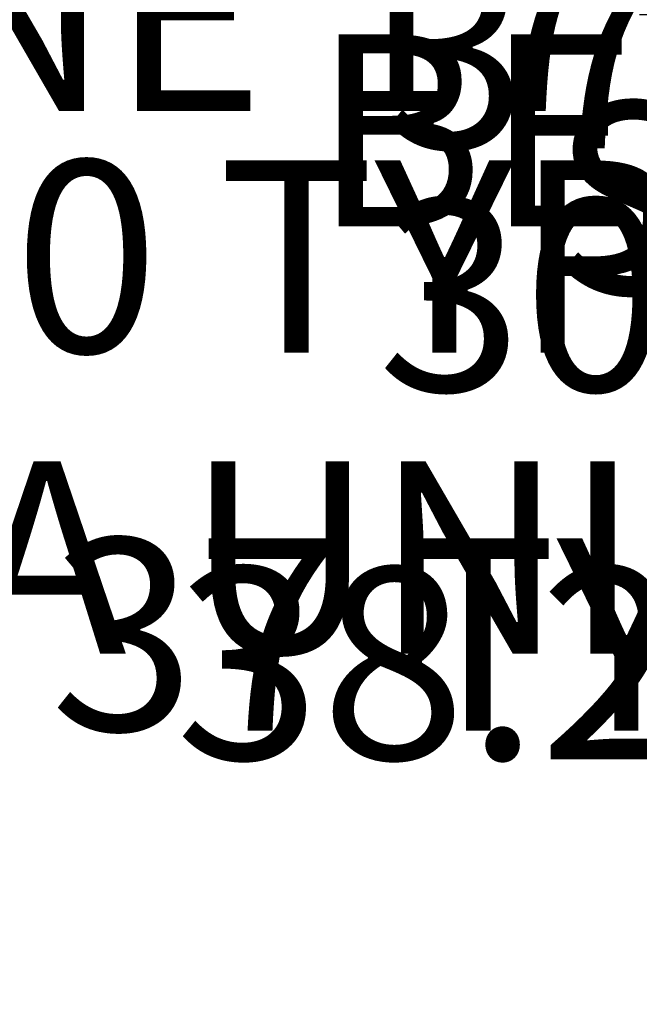
# Model space of a CAD drawing. Units: inches. Extents: x -307 to 2141, y -58 to 895.
# Tile 2 of 28: x 237 to 469, y -58 to 312. Entities that reach past the tile are written whole.
import ezdxf

# ---------------------------------------------------------------- set-up
doc = ezdxf.new("R2010")
doc.units = ezdxf.units.IN
doc.header["$MEASUREMENT"] = 0
doc.layers.add('A-ANNO-DIMS', color=2, linetype='Continuous', lineweight=18)
doc.styles.get("Standard").update_dxf_attribs({"font": 'arial.ttf'})
doc.dimstyles.get("Standard").update_dxf_attribs({"dimtxt": 72, "dimasz": 48, "dimexe": 0.18, "dimexo": 0.0625, "dimgap": 0.09, "dimtad": 0, "dimtih": 1, "dimtoh": 1, "dimdec": 0, "dimrnd": 48, "dimzin": 0, "dimdsep": 46, "dimlunit": 3, "dimtxsty": 'Standard', "dimcen": 0.09, "dimadec": 0, "dimazin": 0, "dimtfac": 1, "dimtdec": 0, "dimtofl": 0, "dimtmove": 0, "dimatfit": 3, "dimfxl": 1, "dimtolj": 1, "dimtzin": 0, "dimarcsym": 0})

# ---------------------------------------------------------------- blocks, each defined once
blk = doc.blocks.new('*D28')
at = {"layer": 'A-ANNO-DIMS', "color": 0, "lineweight": -2, "transparency": 16777216}
for p, q in [((795.36, 433.55), (777.92, 433.55)), ((778.1, 385.55), (778.1, 366.07)), ((795.36, 318.07), (777.92, 318.07)), ((778.1, 318.07), (778.1, 270.07)), ((778.1, 270.07), (730.1, 270.07))]:
    blk.add_line(p, q, dxfattribs=at)
at = {"layer": 'A-ANNO-DIMS', "color": 0, "transparency": 16777216}
for points in [[(770.1, 385.55), (786.1, 385.55), (778.1, 433.55)], [(770.1, 366.07), (786.1, 366.07), (778.1, 318.07)]]:
    blk.add_solid(points, dxfattribs=at)
at = {"layer": 'Defpoints', "color": 0, "transparency": 16777216}
for p in [(795.42, 433.55), (778.1, 318.07), (795.42, 318.07)]:
    blk.add_point(p, dxfattribs=at)
at = {"layer": 'A-ANNO-DIMS', "color": 0, "transparency": 16777216, "insert": (534.42, 270.07), "char_height": 72, "attachment_point": 5}
blk.add_mtext('\\A1;BED 115', dxfattribs=at)
blk = doc.blocks.new('*D36')
at = {"layer": 'A-ANNO-DIMS', "color": 0, "lineweight": -2, "transparency": 16777216}
for p, q in [((871.71, 562.4), (871.76, 610.4)), ((876.55, 514.4), (871.47, 514.4)), ((876.51, 481.35), (871.44, 481.36)), ((871.56, 433.36), (871.51, 385.36)), ((871.51, 385.36), (823.51, 385.36))]:
    blk.add_line(p, q, dxfattribs=at)
at = {"layer": 'A-ANNO-DIMS', "color": 0, "transparency": 16777216}
for points in [[(863.71, 562.41), (879.71, 562.4), (871.65, 514.4)], [(863.56, 433.37), (879.56, 433.35), (871.62, 481.36)]]:
    blk.add_solid(points, dxfattribs=at)
at = {"layer": 'Defpoints', "color": 0, "transparency": 16777216}
for p in [(876.61, 514.4), (871.62, 481.36), (876.57, 481.35)]:
    blk.add_point(p, dxfattribs=at)
at = {"layer": 'A-ANNO-DIMS', "color": 0, "transparency": 16777216, "insert": (548.95, 385.36), "char_height": 72, "attachment_point": 5}
blk.add_mtext('\\A1;WC 33 TYP.', dxfattribs=at)
blk = doc.blocks.new('*D38')
at = {"layer": 'A-ANNO-DIMS', "color": 0, "lineweight": -2, "transparency": 16777216}
for p, q in [((598.5, 222.79), (550.5, 222.79)), ((646.5, 213.85), (646.5, 222.97)), ((706.5, 213.85), (706.5, 222.97)), ((754.5, 222.79), (802.5, 222.79))]:
    blk.add_line(p, q, dxfattribs=at)
at = {"layer": 'A-ANNO-DIMS', "color": 0, "transparency": 16777216}
for points in [[(598.5, 230.79), (598.5, 214.79), (646.5, 222.79)], [(754.5, 230.79), (754.5, 214.79), (706.5, 222.79)]]:
    blk.add_solid(points, dxfattribs=at)
at = {"layer": 'Defpoints', "color": 0, "transparency": 16777216}
for p in [(646.5, 222.79), (646.5, 213.79), (706.5, 213.79)]:
    blk.add_point(p, dxfattribs=at)
at = {"layer": 'A-ANNO-DIMS', "color": 0, "transparency": 16777216, "insert": (97.26, 222.79), "char_height": 72, "attachment_point": 5}
blk.add_mtext('\\A1;LOVESEAT 60 TYP.', dxfattribs=at)
blk = doc.blocks.new('*D39')
at = {"layer": 'A-ANNO-DIMS', "color": 0, "lineweight": -2, "transparency": 16777216}
for p, q in [((637.5, 261.79), (637.5, 309.79)), ((646.43, 213.79), (637.32, 213.79)), ((646.43, 177.12), (637.32, 177.12)), ((637.5, 129.12), (637.5, 81.12)), ((637.5, 81.12), (589.5, 81.12))]:
    blk.add_line(p, q, dxfattribs=at)
at = {"layer": 'A-ANNO-DIMS', "color": 0, "transparency": 16777216}
for points in [[(629.5, 261.79), (645.5, 261.79), (637.5, 213.79)], [(629.5, 129.12), (645.5, 129.12), (637.5, 177.12)]]:
    blk.add_solid(points, dxfattribs=at)
at = {"layer": 'Defpoints', "color": 0, "transparency": 16777216}
for p in [(646.5, 213.79), (637.5, 177.12), (646.5, 177.12)]:
    blk.add_point(p, dxfattribs=at)
at = {"layer": 'A-ANNO-DIMS', "color": 0, "transparency": 16777216, "insert": (414.2, 81.12), "char_height": 72, "attachment_point": 5}
blk.add_mtext('\\A1;37 TYP.', dxfattribs=at)
blk = doc.blocks.new('*D48')
at = {"layer": 'A-ANNO-DIMS', "color": 0, "lineweight": -2, "transparency": 16777216}
for p, q in [((724, 313.98), (724, 361.98)), ((732.94, 265.98), (723.82, 265.98)), ((732.94, 205.98), (723.82, 205.98)), ((724, 157.98), (724, 109.98)), ((724, 109.98), (676, 109.98))]:
    blk.add_line(p, q, dxfattribs=at)
at = {"layer": 'A-ANNO-DIMS', "color": 0, "transparency": 16777216}
for points in [[(716, 313.98), (732, 313.98), (724, 265.98)], [(716, 157.98), (732, 157.98), (724, 205.98)]]:
    blk.add_solid(points, dxfattribs=at)
at = {"layer": 'Defpoints', "color": 0, "transparency": 16777216}
for p in [(733, 265.98), (724, 205.98), (733, 205.98)]:
    blk.add_point(p, dxfattribs=at)
at = {"layer": 'A-ANNO-DIMS', "color": 0, "transparency": 16777216, "insert": (321.56, 109.98), "char_height": 72, "attachment_point": 5}
blk.add_mtext('\\A1;MEDIA UNIT 60', dxfattribs=at)
blk = doc.blocks.new('*D50')
at = {"layer": 'A-ANNO-DIMS', "color": 0, "lineweight": -2, "transparency": 16777216}
for p, q in [((565.34, 315.8), (565.34, 313.15)), ((582.27, 315.8), (582.27, 313.15)), ((517.34, 313.33), (469.34, 313.33)), ((630.27, 313.33), (678.27, 313.33))]:
    blk.add_line(p, q, dxfattribs=at)
at = {"layer": 'A-ANNO-DIMS', "color": 0, "transparency": 16777216}
for points in [[(517.34, 321.33), (517.34, 305.33), (565.34, 313.33)], [(630.27, 321.33), (630.27, 305.33), (582.27, 313.33)]]:
    blk.add_solid(points, dxfattribs=at)
at = {"layer": 'Defpoints', "color": 0, "transparency": 16777216}
for p in [(565.34, 315.87), (582.27, 315.87), (565.34, 313.33)]:
    blk.add_point(p, dxfattribs=at)
at = {"layer": 'A-ANNO-DIMS', "color": 0, "transparency": 16777216, "insert": (226.65, 313.33), "char_height": 72, "attachment_point": 5}
blk.add_mtext('\\A1;PHONE 17', dxfattribs=at)
blk = doc.blocks.new('*D52')
at = {"layer": 'A-ANNO-DIMS', "color": 0, "lineweight": -2, "transparency": 16777216}
for p, q in [((660.21, 554.25), (660.21, 602.25)), ((673.8, 506.25), (660.03, 506.25)), ((673.8, 415.25), (660.03, 415.25)), ((660.21, 367.25), (660.21, 319.25))]:
    blk.add_line(p, q, dxfattribs=at)
at = {"layer": 'A-ANNO-DIMS', "color": 0, "transparency": 16777216}
for points in [[(652.21, 554.25), (668.21, 554.25), (660.21, 506.25)], [(652.21, 367.25), (668.21, 367.25), (660.21, 415.25)]]:
    blk.add_solid(points, dxfattribs=at)
at = {"layer": 'Defpoints', "color": 0, "transparency": 16777216}
for p in [(673.86, 506.25), (660.21, 415.25), (673.86, 415.25)]:
    blk.add_point(p, dxfattribs=at)
at = {"layer": 'A-ANNO-DIMS', "color": 0, "transparency": 16777216, "insert": (660.21, 460.75), "char_height": 72, "attachment_point": 5}
blk.add_mtext('\\A1;DINING SET 91', dxfattribs=at)
blk = doc.blocks.new('*D58')
at = {"layer": 'A-ANNO-DIMS', "color": 0, "lineweight": -2, "transparency": 16777216}
for p, q in [((624.38, 334.8), (624.38, 382.8)), ((611.84, 286.8), (624.56, 286.8)), ((611.84, 202.8), (624.56, 202.8)), ((624.38, 154.8), (624.38, 106.8))]:
    blk.add_line(p, q, dxfattribs=at)
at = {"layer": 'A-ANNO-DIMS', "color": 0, "transparency": 16777216}
for points in [[(616.38, 334.8), (632.38, 334.8), (624.38, 286.8)], [(616.38, 154.8), (632.38, 154.8), (624.38, 202.8)]]:
    blk.add_solid(points, dxfattribs=at)
at = {"layer": 'Defpoints', "color": 0, "transparency": 16777216}
for p in [(611.78, 286.8), (624.38, 286.8), (611.78, 202.8)]:
    blk.add_point(p, dxfattribs=at)
at = {"layer": 'A-ANNO-DIMS', "color": 0, "transparency": 16777216, "insert": (624.38, 244.8), "char_height": 72, "attachment_point": 5}
blk.add_mtext('\\A1;SOFA 84', dxfattribs=at)
blk = doc.blocks.new('*D59')
at = {"layer": 'A-ANNO-DIMS', "color": 0, "lineweight": -2, "transparency": 16777216}
for p, q in [((527.11, 299.4), (479.11, 299.4)), ((575.11, 286.86), (575.11, 299.58)), ((611.78, 286.86), (611.78, 299.58)), ((659.78, 299.4), (707.78, 299.4))]:
    blk.add_line(p, q, dxfattribs=at)
at = {"layer": 'A-ANNO-DIMS', "color": 0, "transparency": 16777216}
for points in [[(527.11, 307.4), (527.11, 291.4), (575.11, 299.4)], [(659.78, 307.4), (659.78, 291.4), (611.78, 299.4)]]:
    blk.add_solid(points, dxfattribs=at)
at = {"layer": 'Defpoints', "color": 0, "transparency": 16777216}
for p in [(575.11, 299.4), (575.11, 286.8), (611.78, 286.8)]:
    blk.add_point(p, dxfattribs=at)
at = {"layer": 'A-ANNO-DIMS', "color": 0, "transparency": 16777216, "insert": (427.48, 299.4), "char_height": 72, "attachment_point": 5}
blk.add_mtext('\\A1;37', dxfattribs=at)
blk = doc.blocks.new('*D64')
at = {"layer": 'A-ANNO-DIMS', "color": 0, "lineweight": -2, "transparency": 16777216}
for p, q in [((556.27, 691.34), (524.95, 691.34)), ((525.13, 643.34), (525.13, 465.69)), ((525.13, 214.34), (525.13, 391.99)), ((556.27, 166.34), (524.95, 166.34))]:
    blk.add_line(p, q, dxfattribs=at)
at = {"layer": 'A-ANNO-DIMS', "color": 0, "transparency": 16777216}
for points in [[(517.13, 643.34), (533.13, 643.34), (525.13, 691.34)], [(517.13, 214.34), (533.13, 214.34), (525.13, 166.34)]]:
    blk.add_solid(points, dxfattribs=at)
at = {"layer": 'Defpoints', "color": 0, "transparency": 16777216}
for p in [(525.13, 691.34), (556.34, 691.34), (556.34, 166.34)]:
    blk.add_point(p, dxfattribs=at)
at = {"layer": 'A-ANNO-DIMS', "color": 0, "transparency": 16777216, "insert": (525.13, 428.84), "char_height": 72, "attachment_point": 5}
blk.add_mtext('\\A1;525', dxfattribs=at)
blk = doc.blocks.new('*D65')
at = {"layer": 'A-ANNO-DIMS', "color": 0, "lineweight": -2, "transparency": 16777216}
for p, q in [((587.54, 252.57), (587.54, 300.57)), ((556.4, 204.57), (587.72, 204.57)), ((556.4, 166.34), (587.72, 166.34)), ((587.54, 118.34), (587.54, 70.34)), ((587.54, 70.34), (539.54, 70.34))]:
    blk.add_line(p, q, dxfattribs=at)
at = {"layer": 'A-ANNO-DIMS', "color": 0, "transparency": 16777216}
for points in [[(579.54, 252.57), (595.54, 252.57), (587.54, 204.57)], [(579.54, 118.34), (595.54, 118.34), (587.54, 166.34)]]:
    blk.add_solid(points, dxfattribs=at)
at = {"layer": 'Defpoints', "color": 0, "transparency": 16777216}
for p in [(556.34, 204.57), (556.34, 166.34), (587.54, 166.34)]:
    blk.add_point(p, dxfattribs=at)
at = {"layer": 'A-ANNO-DIMS', "color": 0, "transparency": 16777216, "insert": (417.99, 70.34), "char_height": 72, "attachment_point": 5}
blk.add_mtext('\\A1;38.23', dxfattribs=at)
blk = doc.blocks.new('*D66')
at = {"layer": 'A-ANNO-DIMS', "color": 0, "lineweight": -2, "transparency": 16777216}
for p, q in [((525.13, 382.34), (525.13, 430.34)), ((556.27, 334.34), (524.95, 334.34)), ((565.27, 304.34), (524.95, 304.34)), ((525.13, 256.34), (525.13, 208.34)), ((525.13, 208.34), (477.13, 208.34))]:
    blk.add_line(p, q, dxfattribs=at)
at = {"layer": 'A-ANNO-DIMS', "color": 0, "transparency": 16777216}
for points in [[(517.13, 382.34), (533.13, 382.34), (525.13, 334.34)], [(517.13, 256.34), (533.13, 256.34), (525.13, 304.34)]]:
    blk.add_solid(points, dxfattribs=at)
at = {"layer": 'Defpoints', "color": 0, "transparency": 16777216}
for p in [(556.34, 334.34), (525.13, 304.34), (565.34, 304.34)]:
    blk.add_point(p, dxfattribs=at)
at = {"layer": 'A-ANNO-DIMS', "color": 0, "transparency": 16777216, "insert": (425.62, 208.34), "char_height": 72, "attachment_point": 5}
blk.add_mtext('\\A1;30', dxfattribs=at)
blk = doc.blocks.new('*D67')
at = {"layer": 'A-ANNO-DIMS', "color": 0, "lineweight": -2, "transparency": 16777216}
for p, q in [((525.13, 496.83), (525.13, 544.83)), ((556.27, 448.83), (524.95, 448.83)), ((556.27, 370.34), (524.95, 370.34)), ((525.13, 322.34), (525.13, 274.34))]:
    blk.add_line(p, q, dxfattribs=at)
at = {"layer": 'A-ANNO-DIMS', "color": 0, "transparency": 16777216}
for points in [[(517.13, 496.83), (533.13, 496.83), (525.13, 448.83)], [(517.13, 322.34), (533.13, 322.34), (525.13, 370.34)]]:
    blk.add_solid(points, dxfattribs=at)
at = {"layer": 'Defpoints', "color": 0, "transparency": 16777216}
for p in [(525.13, 448.83), (556.34, 448.83), (556.34, 370.34)]:
    blk.add_point(p, dxfattribs=at)
at = {"layer": 'A-ANNO-DIMS', "color": 0, "transparency": 16777216, "insert": (525.13, 409.59), "char_height": 72, "attachment_point": 5}
blk.add_mtext('\\A1;78.49', dxfattribs=at)
blk = doc.blocks.new('*D72')
at = {"layer": 'A-ANNO-DIMS', "color": 0, "lineweight": -2, "transparency": 16777216}
for p, q in [((556.34, 91.28), (556.34, 35.96)), ((632.62, 91.28), (632.62, 35.96)), ((508.34, 36.14), (460.34, 36.14)), ((680.62, 36.14), (728.62, 36.14))]:
    blk.add_line(p, q, dxfattribs=at)
at = {"layer": 'A-ANNO-DIMS', "color": 0, "transparency": 16777216}
for points in [[(508.34, 44.14), (508.34, 28.14), (556.34, 36.14)], [(680.62, 44.14), (680.62, 28.14), (632.62, 36.14)]]:
    blk.add_solid(points, dxfattribs=at)
at = {"layer": 'Defpoints', "color": 0, "transparency": 16777216}
for p in [(556.34, 91.34), (632.62, 91.34), (632.62, 36.14)]:
    blk.add_point(p, dxfattribs=at)
at = {"layer": 'A-ANNO-DIMS', "color": 0, "transparency": 16777216, "insert": (849.97, 36.14), "char_height": 72, "attachment_point": 5}
blk.add_mtext('\\A1;76.29', dxfattribs=at)
blk = doc.blocks.new('*D90')
at = {"layer": 'A-ANNO-DIMS', "color": 0, "lineweight": -2, "transparency": 16777216}
for p, q in [((556.34, 166.28), (556.34, 35.96)), ((589.34, 166.28), (589.34, 35.96)), ((508.34, 36.14), (460.34, 36.14)), ((637.34, 36.14), (685.34, 36.14))]:
    blk.add_line(p, q, dxfattribs=at)
at = {"layer": 'A-ANNO-DIMS', "color": 0, "transparency": 16777216}
for points in [[(508.34, 44.14), (508.34, 28.14), (556.34, 36.14)], [(637.34, 44.14), (637.34, 28.14), (589.34, 36.14)]]:
    blk.add_solid(points, dxfattribs=at)
at = {"layer": 'Defpoints', "color": 0, "transparency": 16777216}
for p in [(556.34, 166.34), (589.34, 166.34), (589.34, 36.14)]:
    blk.add_point(p, dxfattribs=at)
at = {"layer": 'A-ANNO-DIMS', "color": 0, "transparency": 16777216, "insert": (736.97, 36.14), "char_height": 72, "attachment_point": 5}
blk.add_mtext('\\A1;33', dxfattribs=at)

msp = doc.modelspace()

# ---------------------------------------------------------------- dimensions: what is measured, and where the dimension line sits
at = {"layer": 'A-ANNO-DIMS'}
for base, p1, p2, angle, override, picture, middle in [((525.1318, 691.3408), (556.3358, 166.3408), (556.3358, 691.3408), 90, {"dimdec": 0, "dimlfac": 1, "dimrnd": 0, "dimzin": 0, "dimdsep": 46, "dimlunit": 2}, '*D64', (525.1318, 428.8408)), ((525.1318, 448.8333), (556.3358, 370.3416), (556.3358, 448.8333), 90, {"dimdec": 2, "dimlfac": 1, "dimrnd": 0, "dimzin": 0, "dimdsep": 46, "dimlunit": 2}, '*D67', (525.1318, 409.5874)), ((525.1318, 304.3408), (556.3358, 334.3416), (565.3358, 304.3408), 90, {"dimdec": 0, "dimlfac": 1, "dimrnd": 0, "dimzin": 0, "dimdsep": 46, "dimlunit": 2}, '*D66', (425.6203, 208.3408)), ((575.1104, 299.3976), (611.777, 286.7976), (575.1104, 286.7976), 180, {"dimdec": 0, "dimlfac": 1, "dimrnd": 0, "dimzin": 0, "dimdsep": 46, "dimlunit": 2}, '*D59', (427.476, 299.3976)), ((587.5398, 166.3408), (556.3358, 204.574), (556.3358, 166.3408), 270, {"dimdec": 2, "dimlfac": 1, "dimrnd": 0, "dimzin": 0, "dimdsep": 46, "dimlunit": 2}, '*D65', (417.9928, 70.3408))]:
    dim = msp.add_linear_dim(base=base, p1=p1, p2=p2, angle=angle, dimstyle='Standard', override=override, dxfattribs=at)
    dim.commit()
    dim.dimension.update_dxf_attribs({"geometry": picture, "text_midpoint": middle})
for base, p1, p2, angle, text, picture, middle in [((660.2083, 415.2485), (673.8583, 506.2485), (673.8583, 415.2485), 270, 'DINING SET <>', '*D52', (660.2083, 460.7485)), ((871.6167, 481.3581), (876.6106, 514.3988), (876.5736, 481.3526), 269.935892, 'WC <> TYP.', '*D36', (548.95, 385.3582)), ((778.0993, 318.073), (795.4208, 433.5496), (795.4208, 318.073), 270, 'BED <>', '*D28', (534.4158, 270.073)), ((565.3358, 313.3263), (582.2714, 315.8666), (565.3358, 315.8666), 180, 'PHONE <>', '*D50', (226.651, 313.3263)), ((646.4965, 222.7908), (706.4965, 213.7908), (646.4965, 213.7908), 180, 'LOVESEAT <> TYP.', '*D38', (97.2632, 222.7908)), ((624.377, 286.7976), (611.777, 202.7976), (611.777, 286.7976), 90, 'SOFA <>', '*D58', (624.377, 244.7976)), ((724.0025, 205.9815), (733.0025, 265.9815), (733.0025, 205.9815), 270, 'MEDIA UNIT <>', '*D48', (321.5605, 109.9815)), ((637.4965, 177.1242), (646.4965, 213.7908), (646.4965, 177.1242), 270, '<> TYP.', '*D39', (414.195, 81.1242))]:
    dim = msp.add_linear_dim(base=base, p1=p1, p2=p2, angle=angle, text=text, dimstyle='Standard', override={"dimdec": 0, "dimlfac": 1, "dimrnd": 0, "dimzin": 0, "dimdsep": 46, "dimlunit": 2}, dxfattribs=at)
    dim.commit()
    dim.dimension.update_dxf_attribs({"geometry": picture, "text_midpoint": middle})
for base, p1, p2, override, picture, middle in [((589.3358, 36.1368), (556.3358, 166.3408), (589.3358, 166.3408), {"dimdec": 0, "dimlfac": 1, "dimrnd": 0, "dimzin": 0, "dimdsep": 46, "dimlunit": 2}, '*D90', (736.9702, 36.1368)), ((632.6211, 36.1368), (556.3358, 91.3408), (632.6211, 91.3408), {"dimdec": 2, "dimlfac": 1, "dimrnd": 0, "dimzin": 0, "dimdsep": 46, "dimlunit": 2}, '*D72', (849.9716, 36.1368))]:
    dim = msp.add_linear_dim(base=base, p1=p1, p2=p2, dimstyle='Standard', override=override, dxfattribs=at)
    dim.commit()
    dim.dimension.update_dxf_attribs({"geometry": picture, "text_midpoint": middle})

doc.saveas('drawing.dxf')
